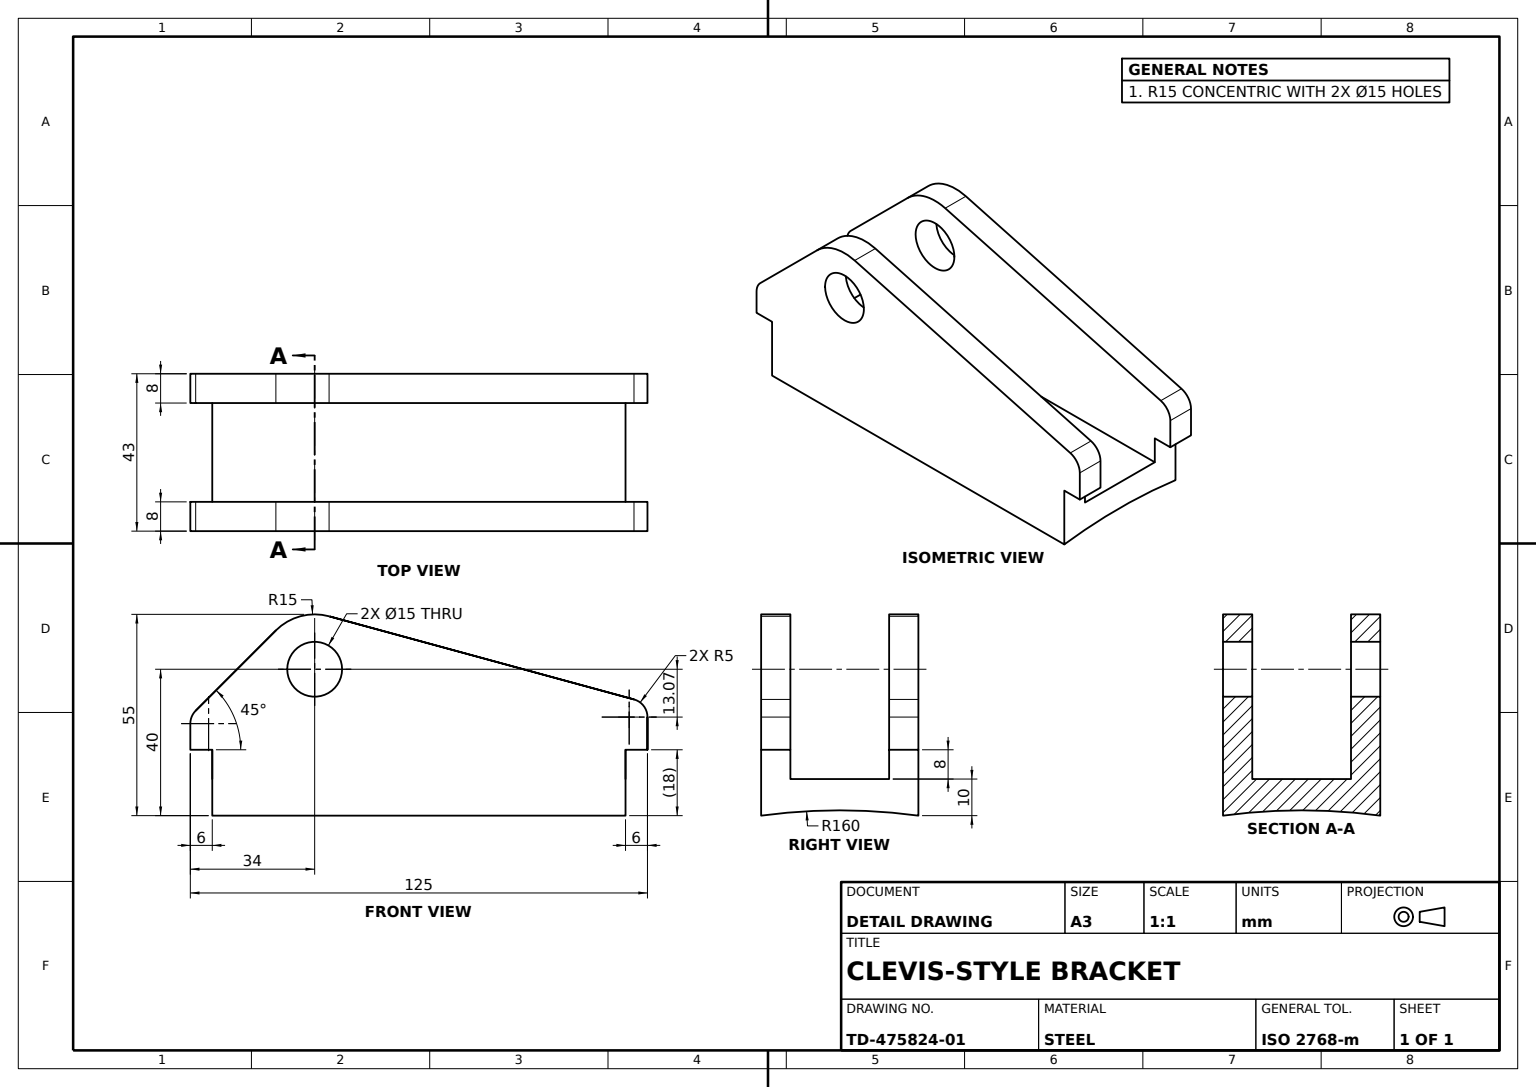
SolidWorks part; units mm, degrees
material "Plain Carbon Steel"
ref_plane "Front Plane" through (0, 0, 0) normal (0, 0, 1) x (1, 0, 0)
ref_plane "Top Plane" through (0, 0, 0) normal (0, 1, 0) x (1, 0, 0)
ref_plane "Right Plane" through (0, 0, 0) normal (1, 0, 0) x (0, 0, -1)
sketch "Clevis Profile Sketch" plane through (0, 0, 0) normal (0, 0, 1) x (1, 0, 0)
  line L0 (0, -49.2033) -> (0, 49.2033) construction
  line L1 (0, 0) -> (111.8279, 0) construction
  line L2 (-10.6066, 10.6066) -> (-32.5355, -11.3223)
  line L3 (3.9434, 14.4724) -> (87.3145, -8.2443)
  line L4 (91, -13.0684) -> (91, -22)
  line L5 (91, -22) -> (85, -22)
  line L6 (85, -22) -> (85, -40)
  line L7 (85, -40) -> (-28, -40)
  line L8 (-28, -40) -> (-28, -22)
  line L9 (-28, -22) -> (-34, -22)
  line L10 (-34, -22) -> (-34, -14.8579)
  line L11 (0, 15) -> (-80.2671, 15)
  circle A0 centre (0, 0) radius 7.5
  arc A1 (3.9434, 14.4724) -> (-10.6066, 10.6066) centre (0, 0) ccw
  arc A2 (91, -13.0684) -> (87.3145, -8.2443) centre (86, -13.0684) ccw
  arc A3 (-34, -14.8579) -> (-32.5355, -11.3223) centre (-29, -14.8579) cw
  point P7 (0, 0)
  point P20 (-34, -18.4289)
  dimension "D1" = 15
  dimension "D2" = 30
  dimension "D11" = 5
  dimension "D3" = 45
  dimension "D4" = 34
  dimension "D5" = 40
  dimension "D6" = 18
  dimension "D7" = 6
  dimension "D8" = 125
  dimension "D9" = 18
  dimension "D10" = 6
  dimension "D12" = 98.4067
  dimension "D13" = 111.8279
  dimension "D14" = 80.2671
  dimension "D15" = 13.0684
extrude "Clevis Body" add sketch "Clevis Profile Sketch" along normal mid plane 43 contours A3 L10 L9 L8 L7 L6 L5 L4 A2 L3 A1 L2 A0
sketch "Clevis Gap Sketch" plane through (85, 0, 0) normal (1, 0, 0) x (0, 0, -1)
  line L0 (-13.5, 15) -> (-13.5, -30)
  line L2 (21.5, 15) -> (-21.5, 15) construction
  line L3 (-13.5, -30) -> (13.5, -30)
  line L4 (13.5, -30) -> (13.5, 15)
  line L5 (-13.5, 15) -> (13.5, 15)
  line L6 (-21.5, -40) -> (21.5, -40) construction
  line L7 (-21.5, 14.4724) -> (-21.5, -8.2443) construction
  line L8 (-21.5, -40) -> (21.5, -40)
  arc A0 (21.5, -40) -> (-21.5, -40) centre (0, -198.5489) ccw
  dimension "D4" = 320
  dimension "D1" = 10
  dimension "D2" = 27
  dimension "D3" = 8
extrude "Clevis Gap Cut" cut sketch "Clevis Gap Sketch" against normal mid plane 373
